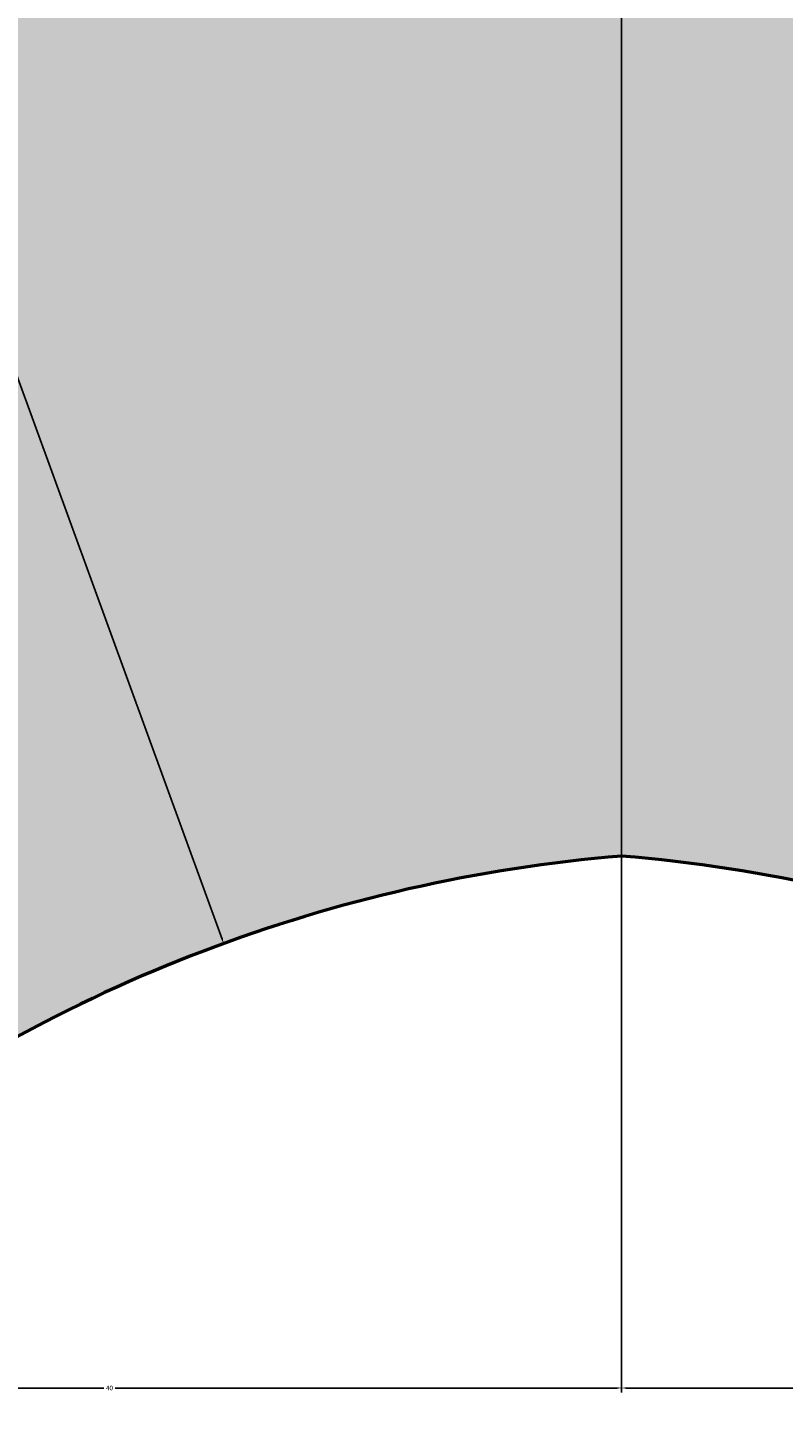
# Model space of a CAD drawing. Units: inches. Extents: x 114 to 236, y -51 to 115.
# Tile 3 of 14: x 152 to 182, y -13 to 41. Entities that reach past the tile are written whole.
import ezdxf

# ---------------------------------------------------------------- set-up
doc = ezdxf.new("R2010")
doc.units = ezdxf.units.IN
doc.header["$MEASUREMENT"] = 0
doc.layers.add('M-DIMS', color=2, linetype='Continuous', lineweight=18)
doc.layers.add('M-OUTL', color=7, linetype='Continuous', lineweight=50)
doc.layers.add('M-HATC', color=7, linetype='Continuous', lineweight=18, true_color=0xffffff)
doc.styles.get("Standard").update_dxf_attribs({"font": 'arial.ttf'})
doc.dimstyles.get("Standard").update_dxf_attribs({"dimtxt": 0.18, "dimasz": 0.18, "dimexe": 0.18, "dimexo": 0.0625, "dimgap": 0.09, "dimtad": 0, "dimtih": 1, "dimtoh": 1, "dimdec": 4, "dimzin": 0, "dimdsep": 46, "dimtxsty": 'Standard', "dimcen": 0.09, "dimadec": 0, "dimazin": 0, "dimtfac": 1, "dimtdec": 4, "dimtofl": 0, "dimtmove": 0, "dimatfit": 3, "dimfxl": 1, "dimtolj": 1, "dimtzin": 0, "dimarcsym": 0})

# ---------------------------------------------------------------- blocks, each defined once
blk = doc.blocks.new('*D3')
at = {"layer": 'Defpoints', "color": 0, "transparency": 16777216}
for p in [(230.229, 115.287), (120.229, 9.307), (230.229, 9.307)]:
    blk.add_point(p, dxfattribs=at)
at = {"layer": 'M-DIMS', "color": 0, "lineweight": -2, "transparency": 16777216}
for p, q in [((120.229, 9.37), (120.229, 115.467)), ((120.409, 115.287), (174.949, 115.287)), ((230.049, 115.287), (175.509, 115.287)), ((230.229, 9.37), (230.229, 115.467))]:
    blk.add_line(p, q, dxfattribs=at)
at = {"layer": 'M-DIMS', "color": 0, "transparency": 16777216}
for points in [[(120.409, 115.317), (120.409, 115.257), (120.229, 115.287)], [(230.049, 115.317), (230.049, 115.257), (230.229, 115.287)]]:
    blk.add_solid(points, dxfattribs=at)
at = {"layer": 'M-DIMS', "color": 0, "transparency": 16777216, "insert": (175.229, 115.287), "char_height": 0.18, "attachment_point": 5}
blk.add_mtext('\\A1;110', dxfattribs=at)
blk = doc.blocks.new('*D4')
at = {"layer": 'Defpoints', "color": 0, "transparency": 16777216}
for p in [(114.249, 109.307), (175.229, 109.307), (135.229, -5.693)]:
    blk.add_point(p, dxfattribs=at)
at = {"layer": 'M-DIMS', "color": 0, "lineweight": -2, "transparency": 16777216}
for p, q in [((175.166, 109.307), (114.069, 109.307)), ((114.249, 109.127), (114.249, 51.989)), ((114.249, -5.513), (114.249, 51.625)), ((135.166, -5.693), (114.069, -5.693))]:
    blk.add_line(p, q, dxfattribs=at)
at = {"layer": 'M-DIMS', "color": 0, "transparency": 16777216}
for points in [[(114.219, 109.127), (114.279, 109.127), (114.249, 109.307)], [(114.219, -5.513), (114.279, -5.513), (114.249, -5.693)]]:
    blk.add_solid(points, dxfattribs=at)
at = {"layer": 'M-DIMS', "color": 0, "transparency": 16777216, "insert": (114.249, 51.807), "char_height": 0.18, "attachment_point": 5}
blk.add_mtext('\\A1;115', dxfattribs=at)
blk = doc.blocks.new('*D5')
at = {"layer": 'Defpoints', "color": 0, "transparency": 16777216}
for p in [(175.229, 79.307), (135.229, 9.307), (175.229, -11.673)]:
    blk.add_point(p, dxfattribs=at)
at = {"layer": 'M-DIMS', "color": 0, "lineweight": -2, "transparency": 16777216}
for p, q in [((175.229, 79.245), (175.229, -11.853)), ((135.229, 9.245), (135.229, -11.853)), ((135.409, -11.673), (155.006, -11.673)), ((175.049, -11.673), (155.451, -11.673))]:
    blk.add_line(p, q, dxfattribs=at)
at = {"layer": 'M-DIMS', "color": 0, "transparency": 16777216}
for points in [[(135.409, -11.643), (135.409, -11.703), (135.229, -11.673)], [(175.049, -11.643), (175.049, -11.703), (175.229, -11.673)]]:
    blk.add_solid(points, dxfattribs=at)
at = {"layer": 'M-DIMS', "color": 0, "transparency": 16777216, "insert": (155.229, -11.673), "char_height": 0.18, "attachment_point": 5}
blk.add_mtext('\\A1;40', dxfattribs=at)
blk = doc.blocks.new('*D6')
at = {"layer": 'Defpoints', "color": 0, "transparency": 16777216}
for p in [(175.229, 79.307), (215.229, 9.307), (215.229, -11.673)]:
    blk.add_point(p, dxfattribs=at)
at = {"layer": 'M-DIMS', "color": 0, "lineweight": -2, "transparency": 16777216}
for p, q in [((175.229, 79.245), (175.229, -11.853)), ((215.229, 9.245), (215.229, -11.853)), ((175.409, -11.673), (195.006, -11.673)), ((215.049, -11.673), (195.451, -11.673))]:
    blk.add_line(p, q, dxfattribs=at)
at = {"layer": 'M-DIMS', "color": 0, "transparency": 16777216}
for points in [[(175.409, -11.643), (175.409, -11.703), (175.229, -11.673)], [(215.049, -11.643), (215.049, -11.703), (215.229, -11.673)]]:
    blk.add_solid(points, dxfattribs=at)
at = {"layer": 'M-DIMS', "color": 0, "transparency": 16777216, "insert": (195.229, -11.673), "char_height": 0.18, "attachment_point": 5}
blk.add_mtext('\\A1;40', dxfattribs=at)
blk = doc.blocks.new('*D7')
at = {"layer": 'Defpoints', "color": 0, "transparency": 16777216}
for p in [(175.229, 79.307), (236.209, 79.307), (215.229, 9.307)]:
    blk.add_point(p, dxfattribs=at)
at = {"layer": 'M-DIMS', "color": 0, "lineweight": -2, "transparency": 16777216}
for p, q in [((175.291, 79.307), (236.389, 79.307)), ((236.209, 79.127), (236.209, 44.489)), ((236.209, 9.487), (236.209, 44.125)), ((215.291, 9.307), (236.389, 9.307))]:
    blk.add_line(p, q, dxfattribs=at)
at = {"layer": 'M-DIMS', "color": 0, "transparency": 16777216}
for points in [[(236.179, 79.127), (236.239, 79.127), (236.209, 79.307)], [(236.179, 9.487), (236.239, 9.487), (236.209, 9.307)]]:
    blk.add_solid(points, dxfattribs=at)
at = {"layer": 'M-DIMS', "color": 0, "transparency": 16777216, "insert": (236.209, 44.307), "char_height": 0.18, "attachment_point": 5}
blk.add_mtext('\\A1;70', dxfattribs=at)
blk = doc.blocks.new('*D14')
at = {"layer": 'Defpoints', "color": 0, "transparency": 16777216}
for p in [(159.689, 5.682), (180.229, -50.693)]:
    blk.add_point(p, dxfattribs=at)
at = {"layer": 'M-DIMS', "color": 0, "lineweight": -2, "transparency": 16777216}
for p, q in [((147.185, 39.507), (147.365, 39.507)), ((147.365, 39.507), (159.627, 5.851)), ((180.139, -50.693), (180.319, -50.693)), ((180.229, -50.783), (180.229, -50.603))]:
    blk.add_line(p, q, dxfattribs=at)
at = {"layer": 'M-DIMS', "color": 0, "transparency": 16777216}
blk.add_solid([(159.655, 5.861), (159.599, 5.841), (159.689, 5.682)], dxfattribs=at)
at = {"layer": 'M-DIMS', "color": 0, "transparency": 16777216, "insert": (146.685, 39.507), "char_height": 0.18, "attachment_point": 5}
blk.add_mtext('\\A1;2X R60', dxfattribs=at)

msp = doc.modelspace()

# ---------------------------------------------------------------- hatches: boundary and pattern name
at = {"layer": 'M-HATC'}
h = msp.add_hatch(color=256, dxfattribs=at)
h.set_gradient(color1=(242, 103, 34), color2=(255, 255, 0), tint=1, name='INVSPHERICAL')
h.paths.add_polyline_path([(145.229, 79.307, -0.060651), (146.105, 86.505), (121.823, 16.038, -0.790743), (150.229, 9.307, -0.236068), (144.229, -2.693, -0.14094), (175.229, 9.098, -0.14094), (206.229, -2.693, -0.236068), (200.229, 9.307, -0.790743), (228.634, 16.038), (204.352, 86.505, -0.060651), (205.229, 79.307, -1)])

# ---------------------------------------------------------------- linework, layer by layer
at = {"layer": 'M-OUTL'}
for centre, start, end in [((180.229, -50.693), 94.78019, 126.8699), ((170.229, -50.693), 53.1301, 85.21981)]:
    msp.add_arc(centre, 60, start, end, dxfattribs=at)

# ---------------------------------------------------------------- dimensions: what is measured, and where the dimension line sits
at = {"layer": 'M-DIMS'}
for base, p1, p2, picture, middle in [((230.229, 115.287), (120.229, 9.307), (230.229, 9.307), '*D3', (175.229, 115.287)), ((175.229, -11.673), (135.229, 9.307), (175.229, 79.307), '*D5', (155.229, -11.673)), ((215.229, -11.673), (175.229, 79.307), (215.229, 9.307), '*D6', (195.229, -11.673))]:
    dim = msp.add_linear_dim(base=base, p1=p1, p2=p2, dimstyle='Standard', override={"dimdec": 0, "dimlfac": 1, "dimrnd": 0, "dimzin": 0, "dimdsep": 46, "dimlunit": 2}, dxfattribs=at)
    dim.commit()
    dim.dimension.update_dxf_attribs({"geometry": picture, "text_midpoint": middle})
for base, p1, p2, picture, middle in [((114.249, 109.307), (135.229, -5.693), (175.229, 109.307), '*D4', (114.249, 51.807)), ((236.209, 79.307), (215.229, 9.307), (175.229, 79.307), '*D7', (236.209, 44.307))]:
    dim = msp.add_linear_dim(base=base, p1=p1, p2=p2, angle=90, dimstyle='Standard', override={"dimdec": 0, "dimlfac": 1, "dimrnd": 0, "dimzin": 0, "dimdsep": 46, "dimlunit": 2}, dxfattribs=at)
    dim.commit()
    dim.dimension.update_dxf_attribs({"geometry": picture, "text_midpoint": middle})
dim = msp.add_radius_dim(center=(180.229, -50.693), mpoint=(159.689, 5.682), text='2X <>', dimstyle='Standard', override={"dimdec": 0, "dimlfac": 1, "dimrnd": 0, "dimzin": 0, "dimdsep": 46, "dimlunit": 2}, dxfattribs=at)
dim.commit()
dim.dimension.update_dxf_attribs({"geometry": '*D14', "text_midpoint": (146.685, 39.507), "dimtype": 164})

doc.saveas('drawing.dxf')
